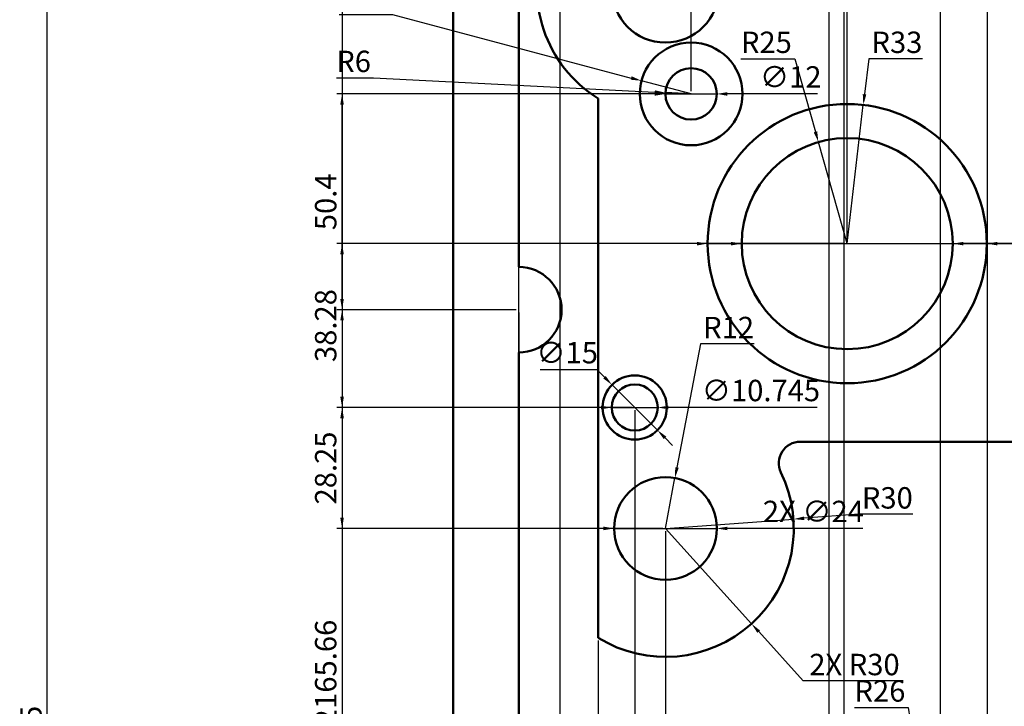
# Model space of a CAD drawing. Units: millimetres. Extents: x 1744 to 2162, y 1763 to 2334.
# Tile 3 of 5: x 1744 to 1975, y 2070 to 2230. Entities that reach past the tile are written whole.
import ezdxf

# ---------------------------------------------------------------- set-up
doc = ezdxf.new("R2010")
doc.units = ezdxf.units.MM
doc.layers.add('M-DIMS', color=2, linetype='Continuous', lineweight=25)
doc.layers.add('M-OUTL', color=7, linetype='Continuous', lineweight=50)
doc.styles.get("Standard").update_dxf_attribs({"font": 'arial.ttf'})
doc.dimstyles.new('ISO-25', dxfattribs={"dimtxt": 5, "dimasz": 2.5, "dimexe": 1.25, "dimexo": 0.625, "dimtad": 1, "dimtoh": 1, "dimdec": 0, "dimtxsty": 'Standard', "dimcen": 2.5, "dimadec": 0, "dimazin": 0, "dimtfac": 1, "dimtdec": 0, "dimtmove": 0, "dimatfit": 3, "dimfxl": 1, "dimarcsym": 0})

# ---------------------------------------------------------------- blocks, each defined once
blk = doc.blocks.new('*D1')
at = {"layer": 'Defpoints', "color": 0, "transparency": 16777216}
for p in [(1750.93, 2301.76), (1845.83, 2301.76), (1863.15, 1826.76)]:
    blk.add_point(p, dxfattribs=at)
at = {"layer": 'M-DIMS', "color": 0, "lineweight": -2, "transparency": 16777216}
for p, q in [((1845.2, 2301.76), (1749.68, 2301.76)), ((1750.93, 1829.26), (1750.93, 2299.26)), ((1862.52, 1826.76), (1749.68, 1826.76))]:
    blk.add_line(p, q, dxfattribs=at)
at = {"layer": 'M-DIMS', "color": 0, "transparency": 16777216}
for points in [[(1750.52, 2299.26), (1751.35, 2299.26), (1750.93, 2301.76)], [(1750.52, 1829.26), (1751.35, 1829.26), (1750.93, 1826.76)]]:
    blk.add_solid(points, dxfattribs=at)
at = {"layer": 'M-DIMS', "color": 0, "transparency": 16777216, "insert": (1747.76, 2064.26), "char_height": 5, "attachment_point": 5, "rotation": 90}
blk.add_mtext('475', dxfattribs=at)
blk = doc.blocks.new('*D8')
at = {"layer": 'Defpoints', "color": 0, "transparency": 16777216}
for p in [(1889.8, 2215.94), (1901.4, 2212.86)]:
    blk.add_point(p, dxfattribs=at)
at = {"layer": 'M-DIMS', "color": 0, "lineweight": -2, "transparency": 16777216}
for p, q in [((1819.12, 2231.4), (1831.64, 2231.4)), ((1831.64, 2231.4), (1887.38, 2216.58)), ((1901.4, 2212.86), (1889.8, 2215.94))]:
    blk.add_line(p, q, dxfattribs=at)
at = {"layer": 'M-DIMS', "color": 0, "transparency": 16777216}
blk.add_solid([(1887.49, 2216.99), (1887.28, 2216.18), (1889.8, 2215.94)], dxfattribs=at)
at = {"layer": 'M-DIMS', "color": 0, "transparency": 16777216, "insert": (1825.07, 2234.54), "char_height": 5, "attachment_point": 5}
blk.add_mtext('R12', dxfattribs=at)
blk = doc.blocks.new('*D9')
at = {"layer": 'Defpoints', "color": 0, "transparency": 16777216}
for p in [(1895.4, 2213.16), (1901.4, 2212.86)]:
    blk.add_point(p, dxfattribs=at)
at = {"layer": 'M-DIMS', "color": 0, "lineweight": -2, "transparency": 16777216}
for p, q in [((1818.49, 2216.64), (1827.18, 2216.64)), ((1827.18, 2216.64), (1892.91, 2213.29)), ((1901.4, 2212.86), (1895.4, 2213.16))]:
    blk.add_line(p, q, dxfattribs=at)
at = {"layer": 'M-DIMS', "color": 0, "transparency": 16777216}
blk.add_solid([(1892.93, 2213.71), (1892.89, 2212.87), (1895.4, 2213.16)], dxfattribs=at)
at = {"layer": 'M-DIMS', "color": 0, "transparency": 16777216, "insert": (1822.52, 2219.81), "char_height": 5, "attachment_point": 5}
blk.add_mtext('R6', dxfattribs=at)
blk = doc.blocks.new('*D10')
at = {"layer": 'Defpoints', "color": 0, "transparency": 16777216}
for p in [(1931.15, 2201.61), (1937.89, 2177.89)]:
    blk.add_point(p, dxfattribs=at)
at = {"layer": 'M-DIMS', "color": 0, "lineweight": -2, "transparency": 16777216}
for p, q in [((1913, 2221.09), (1925.61, 2221.09)), ((1925.61, 2221.09), (1930.47, 2204.01)), ((1937.89, 2177.89), (1931.15, 2201.61))]:
    blk.add_line(p, q, dxfattribs=at)
at = {"layer": 'M-DIMS', "color": 0, "transparency": 16777216}
blk.add_solid([(1930.87, 2204.12), (1930.06, 2203.9), (1931.15, 2201.61)], dxfattribs=at)
at = {"layer": 'M-DIMS', "color": 0, "transparency": 16777216, "insert": (1918.99, 2224.27), "char_height": 5, "attachment_point": 5}
blk.add_mtext('R25', dxfattribs=at)
blk = doc.blocks.new('*D11')
at = {"layer": 'Defpoints', "color": 0, "transparency": 16777216}
for p in [(1941.65, 2210.29), (1937.89, 2177.89)]:
    blk.add_point(p, dxfattribs=at)
at = {"layer": 'M-DIMS', "color": 0, "lineweight": -2, "transparency": 16777216}
for p, q in [((1942.9, 2221.09), (1941.93, 2212.77)), ((1955.47, 2221.09), (1942.9, 2221.09)), ((1937.89, 2177.89), (1941.65, 2210.29))]:
    blk.add_line(p, q, dxfattribs=at)
at = {"layer": 'M-DIMS', "color": 0, "transparency": 16777216}
blk.add_solid([(1941.52, 2212.82), (1942.35, 2212.72), (1941.65, 2210.29)], dxfattribs=at)
at = {"layer": 'M-DIMS', "color": 0, "transparency": 16777216, "insert": (1949.5, 2224.27), "char_height": 5, "attachment_point": 5}
blk.add_mtext('R33', dxfattribs=at)
blk = doc.blocks.new('*D12')
at = {"layer": 'Defpoints', "color": 0, "transparency": 16777216}
for p in [(1897.63, 2123.15), (1895.4, 2111.36)]:
    blk.add_point(p, dxfattribs=at)
at = {"layer": 'M-DIMS', "color": 0, "lineweight": -2, "transparency": 16777216}
for p, q in [((1903.58, 2154.51), (1898.1, 2125.6)), ((1916.1, 2154.51), (1903.58, 2154.51)), ((1895.4, 2111.36), (1897.63, 2123.15))]:
    blk.add_line(p, q, dxfattribs=at)
at = {"layer": 'M-DIMS', "color": 0, "transparency": 16777216}
blk.add_solid([(1897.69, 2125.68), (1898.51, 2125.53), (1897.63, 2123.15)], dxfattribs=at)
at = {"layer": 'M-DIMS', "color": 0, "transparency": 16777216, "insert": (1910.16, 2157.64), "char_height": 5, "attachment_point": 5}
blk.add_mtext('R12', dxfattribs=at)
blk = doc.blocks.new('*D13')
at = {"layer": 'Defpoints', "color": 0, "transparency": 16777216}
for p in [(1925.32, 2113.54), (1895.4, 2111.36)]:
    blk.add_point(p, dxfattribs=at)
at = {"layer": 'M-DIMS', "color": 0, "lineweight": -2, "transparency": 16777216}
for p, q in [((1895.4, 2111.36), (1925.32, 2113.54)), ((1940.67, 2114.67), (1927.81, 2113.73)), ((1953.23, 2114.67), (1940.67, 2114.67))]:
    blk.add_line(p, q, dxfattribs=at)
at = {"layer": 'M-DIMS', "color": 0, "transparency": 16777216}
blk.add_solid([(1927.78, 2114.14), (1927.84, 2113.31), (1925.32, 2113.54)], dxfattribs=at)
at = {"layer": 'M-DIMS', "color": 0, "transparency": 16777216, "insert": (1947.26, 2117.85), "char_height": 5, "attachment_point": 5}
blk.add_mtext('R30', dxfattribs=at)
blk = doc.blocks.new('*D15')
at = {"layer": 'Defpoints', "color": 0, "transparency": 16777216}
for p in [(1955.73, 2046.29), (1959.65, 2021.02)]:
    blk.add_point(p, dxfattribs=at)
at = {"layer": 'M-DIMS', "color": 0, "lineweight": -2, "transparency": 16777216}
for p, q in [((1939.55, 2069.57), (1952.12, 2069.57)), ((1952.12, 2069.57), (1955.35, 2048.77)), ((1959.65, 2021.02), (1955.73, 2046.29))]:
    blk.add_line(p, q, dxfattribs=at)
at = {"layer": 'M-DIMS', "color": 0, "transparency": 16777216}
blk.add_solid([(1955.76, 2048.83), (1954.94, 2048.7), (1955.73, 2046.29)], dxfattribs=at)
at = {"layer": 'M-DIMS', "color": 0, "transparency": 16777216, "insert": (1945.53, 2072.75), "char_height": 5, "attachment_point": 5}
blk.add_mtext('R26', dxfattribs=at)
blk = doc.blocks.new('*D29')
at = {"layer": 'Defpoints', "color": 0, "transparency": 16777216}
for p in [(2052.51, 2327.76), (2052.51, 1966.98), (1937.15, 1938.72)]:
    blk.add_point(p, dxfattribs=at)
at = {"layer": 'M-DIMS', "color": 0, "lineweight": -2, "transparency": 16777216}
for p, q in [((1937.15, 1939.34), (1937.15, 2329.01)), ((2052.51, 1967.6), (2052.51, 2329.01)), ((1939.65, 2327.76), (2050.01, 2327.76))]:
    blk.add_line(p, q, dxfattribs=at)
at = {"layer": 'M-DIMS', "color": 0, "transparency": 16777216}
for points in [[(1939.65, 2328.18), (1939.65, 2327.34), (1937.15, 2327.76)], [(2050.01, 2328.18), (2050.01, 2327.34), (2052.51, 2327.76)]]:
    blk.add_solid(points, dxfattribs=at)
at = {"layer": 'M-DIMS', "color": 0, "transparency": 16777216, "insert": (1994.83, 2330.94), "char_height": 5, "attachment_point": 5}
blk.add_mtext('115.35', dxfattribs=at)
blk = doc.blocks.new('*D30')
at = {"layer": 'Defpoints', "color": 0, "transparency": 16777216}
for p in [(1959.65, 2327.76), (1959.65, 2021.02), (1937.15, 1938.72)]:
    blk.add_point(p, dxfattribs=at)
at = {"layer": 'M-DIMS', "color": 0, "lineweight": -2, "transparency": 16777216}
for p, q in [((1937.15, 1939.34), (1937.15, 2329.01)), ((1959.65, 2021.64), (1959.65, 2329.01)), ((1939.65, 2327.76), (1957.15, 2327.76))]:
    blk.add_line(p, q, dxfattribs=at)
at = {"layer": 'M-DIMS', "color": 0, "transparency": 16777216}
for points in [[(1939.65, 2328.18), (1939.65, 2327.34), (1937.15, 2327.76)], [(1957.15, 2328.18), (1957.15, 2327.34), (1959.65, 2327.76)]]:
    blk.add_solid(points, dxfattribs=at)
at = {"layer": 'M-DIMS', "color": 0, "transparency": 16777216, "insert": (1948.4, 2330.94), "char_height": 5, "attachment_point": 5}
blk.add_mtext('22.5', dxfattribs=at)
blk = doc.blocks.new('*D34')
at = {"layer": 'Defpoints', "color": 0, "transparency": 16777216}
for p in [(2003.18, 2327.76), (2003.18, 2221.73), (1937.89, 2177.89)]:
    blk.add_point(p, dxfattribs=at)
at = {"layer": 'M-DIMS', "color": 0, "lineweight": -2, "transparency": 16777216}
for p, q in [((1937.89, 2178.51), (1937.89, 2329.01)), ((2003.18, 2222.36), (2003.18, 2329.01)), ((1940.39, 2327.76), (2000.68, 2327.76))]:
    blk.add_line(p, q, dxfattribs=at)
at = {"layer": 'M-DIMS', "color": 0, "transparency": 16777216}
for points in [[(1940.39, 2328.18), (1940.39, 2327.34), (1937.89, 2327.76)], [(2000.68, 2328.18), (2000.68, 2327.34), (2003.18, 2327.76)]]:
    blk.add_solid(points, dxfattribs=at)
at = {"layer": 'M-DIMS', "color": 0, "transparency": 16777216, "insert": (1970.53, 2330.94), "char_height": 5, "attachment_point": 5}
blk.add_mtext('65.29', dxfattribs=at)
blk = doc.blocks.new('*D36')
at = {"layer": 'Defpoints', "color": 0, "transparency": 16777216}
for p in [(1937.89, 2327.76), (1901.4, 2212.86), (1937.89, 2177.89)]:
    blk.add_point(p, dxfattribs=at)
at = {"layer": 'M-DIMS', "color": 0, "lineweight": -2, "transparency": 16777216}
for p, q in [((1901.4, 2213.48), (1901.4, 2329.01)), ((1937.89, 2178.51), (1937.89, 2329.01)), ((1903.9, 2327.76), (1935.39, 2327.76))]:
    blk.add_line(p, q, dxfattribs=at)
at = {"layer": 'M-DIMS', "color": 0, "transparency": 16777216}
for points in [[(1903.9, 2328.18), (1903.9, 2327.34), (1901.4, 2327.76)], [(1935.39, 2328.18), (1935.39, 2327.34), (1937.89, 2327.76)]]:
    blk.add_solid(points, dxfattribs=at)
at = {"layer": 'M-DIMS', "color": 0, "transparency": 16777216, "insert": (1919.64, 2330.94), "char_height": 5, "attachment_point": 5}
blk.add_mtext('36.49', dxfattribs=at)
blk = doc.blocks.new('*D37')
at = {"layer": 'Defpoints', "color": 0, "transparency": 16777216}
for p in [(1861.12, 2162.45), (1888.22, 2139.61), (1888.22, 1800.76)]:
    blk.add_point(p, dxfattribs=at)
at = {"layer": 'M-DIMS', "color": 0, "lineweight": -2, "transparency": 16777216}
for p, q in [((1861.12, 2161.83), (1861.12, 1799.51)), ((1888.22, 2138.98), (1888.22, 1799.51)), ((1863.62, 1800.76), (1885.72, 1800.76))]:
    blk.add_line(p, q, dxfattribs=at)
at = {"layer": 'M-DIMS', "color": 0, "transparency": 16777216}
for points in [[(1863.62, 1801.18), (1863.62, 1800.34), (1861.12, 1800.76)], [(1885.72, 1801.18), (1885.72, 1800.34), (1888.22, 1800.76)]]:
    blk.add_solid(points, dxfattribs=at)
at = {"layer": 'M-DIMS', "color": 0, "transparency": 16777216, "insert": (1874.67, 1803.9), "char_height": 5, "attachment_point": 5}
blk.add_mtext('27.1', dxfattribs=at)
blk = doc.blocks.new('*D39')
at = {"layer": 'Defpoints', "color": 0, "transparency": 16777216}
for p in [(1819.83, 2212.86), (1901.4, 2212.86), (1861.12, 2162.45)]:
    blk.add_point(p, dxfattribs=at)
at = {"layer": 'M-DIMS', "color": 0, "lineweight": -2, "transparency": 16777216}
for p, q in [((1900.77, 2212.86), (1818.58, 2212.86)), ((1819.83, 2164.95), (1819.83, 2210.36)), ((1860.5, 2162.45), (1818.58, 2162.45))]:
    blk.add_line(p, q, dxfattribs=at)
at = {"layer": 'M-DIMS', "color": 0, "transparency": 16777216}
for points in [[(1819.41, 2210.36), (1820.24, 2210.36), (1819.83, 2212.86)], [(1819.41, 2164.95), (1820.24, 2164.95), (1819.83, 2162.45)]]:
    blk.add_solid(points, dxfattribs=at)
at = {"layer": 'M-DIMS', "color": 0, "transparency": 16777216, "insert": (1816.65, 2187.66), "char_height": 5, "attachment_point": 5, "rotation": 90}
blk.add_mtext('50.4', dxfattribs=at)
blk = doc.blocks.new('*D40')
at = {"layer": 'Defpoints', "color": 0, "transparency": 16777216}
for p in [(1937.89, 2177.89), (2091.83, 2177.89), (2003.18, 2145.53)]:
    blk.add_point(p, dxfattribs=at)
at = {"layer": 'M-DIMS', "color": 0, "lineweight": -2, "transparency": 16777216}
for p, q in [((1938.51, 2177.89), (2093.08, 2177.89)), ((2091.83, 2148.03), (2091.83, 2175.39)), ((2003.8, 2145.53), (2093.08, 2145.53))]:
    blk.add_line(p, q, dxfattribs=at)
at = {"layer": 'M-DIMS', "color": 0, "transparency": 16777216}
for points in [[(2091.41, 2175.39), (2092.24, 2175.39), (2091.83, 2177.89)], [(2091.41, 2148.03), (2092.24, 2148.03), (2091.83, 2145.53)]]:
    blk.add_solid(points, dxfattribs=at)
at = {"layer": 'M-DIMS', "color": 0, "transparency": 16777216, "insert": (2088.65, 2161.71), "char_height": 5, "attachment_point": 5, "rotation": 90}
blk.add_mtext('32.36', dxfattribs=at)
blk = doc.blocks.new('*D41')
at = {"layer": 'Defpoints', "color": 0, "transparency": 16777216}
for p in [(1937.89, 2177.89), (1819.83, 2139.61), (1888.22, 2139.61)]:
    blk.add_point(p, dxfattribs=at)
at = {"layer": 'M-DIMS', "color": 0, "lineweight": -2, "transparency": 16777216}
for p, q in [((1937.26, 2177.89), (1818.58, 2177.89)), ((1819.83, 2175.39), (1819.83, 2142.11)), ((1887.6, 2139.61), (1818.58, 2139.61))]:
    blk.add_line(p, q, dxfattribs=at)
at = {"layer": 'M-DIMS', "color": 0, "transparency": 16777216}
for points in [[(1819.41, 2175.39), (1820.24, 2175.39), (1819.83, 2177.89)], [(1819.41, 2142.11), (1820.24, 2142.11), (1819.83, 2139.61)]]:
    blk.add_solid(points, dxfattribs=at)
at = {"layer": 'M-DIMS', "color": 0, "transparency": 16777216, "insert": (1816.65, 2158.75), "char_height": 5, "attachment_point": 5, "rotation": 90}
blk.add_mtext('38.28', dxfattribs=at)
blk = doc.blocks.new('*D42')
at = {"layer": 'Defpoints', "color": 0, "transparency": 16777216}
for p in [(1888.22, 2139.61), (1819.83, 2111.36), (1895.4, 2111.36)]:
    blk.add_point(p, dxfattribs=at)
at = {"layer": 'M-DIMS', "color": 0, "lineweight": -2, "transparency": 16777216}
for p, q in [((1887.6, 2139.61), (1818.58, 2139.61)), ((1819.83, 2137.11), (1819.83, 2113.86)), ((1894.77, 2111.36), (1818.58, 2111.36))]:
    blk.add_line(p, q, dxfattribs=at)
at = {"layer": 'M-DIMS', "color": 0, "transparency": 16777216}
for points in [[(1819.41, 2137.11), (1820.24, 2137.11), (1819.83, 2139.61)], [(1819.41, 2113.86), (1820.24, 2113.86), (1819.83, 2111.36)]]:
    blk.add_solid(points, dxfattribs=at)
at = {"layer": 'M-DIMS', "color": 0, "transparency": 16777216, "insert": (1816.65, 2125.48), "char_height": 5, "attachment_point": 5, "rotation": 90}
blk.add_mtext('28.25', dxfattribs=at)
blk = doc.blocks.new('*D46')
at = {"layer": 'Defpoints', "color": 0, "transparency": 16777216}
for p in [(2052.51, 2327.76), (1861.12, 1859.18), (2052.51, 1857.29)]:
    blk.add_point(p, dxfattribs=at)
at = {"layer": 'M-DIMS', "color": 0, "lineweight": -2, "transparency": 16777216}
for p, q in [((1861.12, 1859.81), (1861.12, 2329.01)), ((2052.51, 1857.91), (2052.51, 2329.01)), ((1863.62, 2327.76), (2050.01, 2327.76))]:
    blk.add_line(p, q, dxfattribs=at)
at = {"layer": 'M-DIMS', "color": 0, "transparency": 16777216}
for points in [[(1863.62, 2328.18), (1863.62, 2327.34), (1861.12, 2327.76)], [(2050.01, 2328.18), (2050.01, 2327.34), (2052.51, 2327.76)]]:
    blk.add_solid(points, dxfattribs=at)
at = {"layer": 'M-DIMS', "color": 0, "transparency": 16777216, "insert": (1956.82, 2330.94), "char_height": 5, "attachment_point": 5}
blk.add_mtext('191.4', dxfattribs=at)
blk = doc.blocks.new('*D47')
at = {"layer": 'Defpoints', "color": 0, "transparency": 16777216}
for p in [(1871.12, 2284.44), (1819.83, 1842.43), (1870.79, 1842.43)]:
    blk.add_point(p, dxfattribs=at)
at = {"layer": 'M-DIMS', "color": 0, "lineweight": -2, "transparency": 16777216}
for p, q in [((1870.5, 2284.44), (1818.58, 2284.44)), ((1819.83, 2281.94), (1819.83, 1844.93)), ((1870.17, 1842.43), (1818.58, 1842.43))]:
    blk.add_line(p, q, dxfattribs=at)
at = {"layer": 'M-DIMS', "color": 0, "transparency": 16777216}
for points in [[(1819.41, 2281.94), (1820.24, 2281.94), (1819.83, 2284.44)], [(1819.41, 1844.93), (1820.24, 1844.93), (1819.83, 1842.43)]]:
    blk.add_solid(points, dxfattribs=at)
at = {"layer": 'M-DIMS', "color": 0, "transparency": 16777216, "insert": (1816.69, 2063.44), "char_height": 5, "attachment_point": 5, "rotation": 90}
blk.add_mtext('442', dxfattribs=at)
blk = doc.blocks.new('*D48')
at = {"layer": 'Defpoints', "color": 0, "transparency": 16777216}
for p in [(1861.12, 2327.76), (1861.12, 1859.18), (1845.83, 1856.76)]:
    blk.add_point(p, dxfattribs=at)
at = {"layer": 'M-DIMS', "color": 0, "lineweight": -2, "transparency": 16777216}
for p, q in [((1845.83, 1857.39), (1845.83, 2329.01)), ((1861.12, 1859.81), (1861.12, 2329.01)), ((1848.33, 2327.76), (1858.62, 2327.76)), ((1861.12, 2327.76), (1885.17, 2327.76))]:
    blk.add_line(p, q, dxfattribs=at)
at = {"layer": 'M-DIMS', "color": 0, "transparency": 16777216}
for points in [[(1848.33, 2328.18), (1848.33, 2327.34), (1845.83, 2327.76)], [(1858.62, 2328.18), (1858.62, 2327.34), (1861.12, 2327.76)]]:
    blk.add_solid(points, dxfattribs=at)
at = {"layer": 'M-DIMS', "color": 0, "transparency": 16777216, "insert": (1874.4, 2330.94), "char_height": 5, "attachment_point": 5}
blk.add_mtext('15.298', dxfattribs=at)
blk = doc.blocks.new('*D53')
at = {"layer": 'Defpoints', "color": 0, "transparency": 16777216}
for p in [(1861.12, 2162.45), (1819.83, 1996.79), (1861.12, 1996.79)]:
    blk.add_point(p, dxfattribs=at)
at = {"layer": 'M-DIMS', "color": 0, "lineweight": -2, "transparency": 16777216}
for p, q in [((1860.5, 2162.45), (1818.58, 2162.45)), ((1819.83, 2159.95), (1819.83, 1999.29)), ((1860.5, 1996.79), (1818.58, 1996.79))]:
    blk.add_line(p, q, dxfattribs=at)
at = {"layer": 'M-DIMS', "color": 0, "transparency": 16777216}
for points in [[(1819.41, 2159.95), (1820.24, 2159.95), (1819.83, 2162.45)], [(1819.41, 1999.29), (1820.24, 1999.29), (1819.83, 1996.79)]]:
    blk.add_solid(points, dxfattribs=at)
at = {"layer": 'M-DIMS', "color": 0, "transparency": 16777216, "insert": (1816.65, 2079.62), "char_height": 5, "attachment_point": 5, "rotation": 90}
blk.add_mtext('165.66', dxfattribs=at)
blk = doc.blocks.new('*D60')
at = {"layer": 'Defpoints', "color": 0, "transparency": 16777216}
for p in [(1933.69, 2327.76), (1870.79, 1842.43), (1933.69, 1842.43)]:
    blk.add_point(p, dxfattribs=at)
at = {"layer": 'M-DIMS', "color": 0, "lineweight": -2, "transparency": 16777216}
for p, q in [((1870.79, 1843.06), (1870.79, 2329.01)), ((1933.69, 1843.06), (1933.69, 2329.01)), ((1873.29, 2327.76), (1931.19, 2327.76))]:
    blk.add_line(p, q, dxfattribs=at)
at = {"layer": 'M-DIMS', "color": 0, "transparency": 16777216}
for points in [[(1873.29, 2328.18), (1873.29, 2327.34), (1870.79, 2327.76)], [(1931.19, 2328.18), (1931.19, 2327.34), (1933.69, 2327.76)]]:
    blk.add_solid(points, dxfattribs=at)
at = {"layer": 'M-DIMS', "color": 0, "transparency": 16777216, "insert": (1902.24, 2330.94), "char_height": 5, "attachment_point": 5}
blk.add_mtext('62.9', dxfattribs=at)
blk = doc.blocks.new('*D61')
at = {"layer": 'Defpoints', "color": 0, "transparency": 16777216}
for p in [(1970.69, 2327.76), (1933.69, 1842.43), (1970.69, 1842.43)]:
    blk.add_point(p, dxfattribs=at)
at = {"layer": 'M-DIMS', "color": 0, "lineweight": -2, "transparency": 16777216}
for p, q in [((1933.69, 1843.06), (1933.69, 2329.01)), ((1970.69, 1843.06), (1970.69, 2329.01)), ((1936.19, 2327.76), (1968.19, 2327.76))]:
    blk.add_line(p, q, dxfattribs=at)
at = {"layer": 'M-DIMS', "color": 0, "transparency": 16777216}
for points in [[(1936.19, 2328.18), (1936.19, 2327.34), (1933.69, 2327.76)], [(1968.19, 2328.18), (1968.19, 2327.34), (1970.69, 2327.76)]]:
    blk.add_solid(points, dxfattribs=at)
at = {"layer": 'M-DIMS', "color": 0, "transparency": 16777216, "insert": (1952.19, 2330.94), "char_height": 5, "attachment_point": 5}
blk.add_mtext('37', dxfattribs=at)
blk = doc.blocks.new('*D67')
at = {"layer": 'Defpoints', "color": 0, "transparency": 16777216}
for p in [(1861.12, 2162.45), (1895.4, 2111.36), (1895.4, 1800.76)]:
    blk.add_point(p, dxfattribs=at)
at = {"layer": 'M-DIMS', "color": 0, "lineweight": -2, "transparency": 16777216}
for p, q in [((1861.12, 2161.83), (1861.12, 1799.51)), ((1895.4, 2110.73), (1895.4, 1799.51)), ((1863.62, 1800.76), (1892.9, 1800.76))]:
    blk.add_line(p, q, dxfattribs=at)
at = {"layer": 'M-DIMS', "color": 0, "transparency": 16777216}
for points in [[(1863.62, 1801.18), (1863.62, 1800.34), (1861.12, 1800.76)], [(1892.9, 1801.18), (1892.9, 1800.34), (1895.4, 1800.76)]]:
    blk.add_solid(points, dxfattribs=at)
at = {"layer": 'M-DIMS', "color": 0, "transparency": 16777216, "insert": (1878.26, 1803.94), "char_height": 5, "attachment_point": 5}
blk.add_mtext('34.273', dxfattribs=at)
blk = doc.blocks.new('*D69')
at = {"layer": 'Defpoints', "color": 0, "transparency": 16777216}
for p in [(1861.12, 2162.45), (1879.67, 2085.81), (1861.12, 1800.76)]:
    blk.add_point(p, dxfattribs=at)
at = {"layer": 'M-DIMS', "color": 0, "lineweight": -2, "transparency": 16777216}
for p, q in [((1861.12, 2161.83), (1861.12, 1799.51)), ((1879.67, 2085.19), (1879.67, 1799.51)), ((1877.17, 1800.76), (1863.62, 1800.76))]:
    blk.add_line(p, q, dxfattribs=at)
at = {"layer": 'M-DIMS', "color": 0, "transparency": 16777216}
for points in [[(1863.62, 1801.18), (1863.62, 1800.34), (1861.12, 1800.76)], [(1877.17, 1801.18), (1877.17, 1800.34), (1879.67, 1800.76)]]:
    blk.add_solid(points, dxfattribs=at)
at = {"layer": 'M-DIMS', "color": 0, "transparency": 16777216, "insert": (1870.39, 1803.94), "char_height": 5, "attachment_point": 5}
blk.add_mtext('18.54', dxfattribs=at)
blk = doc.blocks.new('*D74')
at = {"layer": 'Defpoints', "color": 0, "transparency": 16777216}
for p in [(1882.92, 2144.91), (1893.53, 2134.31)]:
    blk.add_point(p, dxfattribs=at)
at = {"layer": 'M-DIMS', "color": 0, "lineweight": -2, "transparency": 16777216}
for p, q in [((1866.12, 2148.45), (1879.38, 2148.45)), ((1879.38, 2148.45), (1881.15, 2146.68)), ((1893.53, 2134.31), (1882.92, 2144.91)), ((1895.3, 2132.54), (1897.06, 2130.77))]:
    blk.add_line(p, q, dxfattribs=at)
at = {"layer": 'M-DIMS', "color": 0, "transparency": 16777216}
for points in [[(1881.45, 2146.97), (1880.86, 2146.39), (1882.92, 2144.91)], [(1895.59, 2132.83), (1895, 2132.24), (1893.53, 2134.31)]]:
    blk.add_solid(points, dxfattribs=at)
at = {"layer": 'M-DIMS', "color": 0, "transparency": 16777216, "insert": (1872.44, 2151.77), "char_height": 5, "attachment_point": 5}
blk.add_mtext('∅15', dxfattribs=at)
blk = doc.blocks.new('*D75')
at = {"layer": 'Defpoints', "color": 0, "transparency": 16777216}
for p in [(1882.85, 2139.61), (1893.6, 2139.61)]:
    blk.add_point(p, dxfattribs=at)
at = {"layer": 'M-DIMS', "color": 0, "lineweight": -2, "transparency": 16777216}
for p, q in [((1880.35, 2139.61), (1877.85, 2139.61)), ((1882.85, 2139.61), (1893.6, 2139.61)), ((1903.98, 2139.61), (1896.1, 2139.61)), ((1930.84, 2139.61), (1903.98, 2139.61))]:
    blk.add_line(p, q, dxfattribs=at)
at = {"layer": 'M-DIMS', "color": 0, "transparency": 16777216}
for points in [[(1880.35, 2140.03), (1880.35, 2139.19), (1882.85, 2139.61)], [(1896.1, 2140.03), (1896.1, 2139.19), (1893.6, 2139.61)]]:
    blk.add_solid(points, dxfattribs=at)
at = {"layer": 'M-DIMS', "color": 0, "transparency": 16777216, "insert": (1917.72, 2142.93), "char_height": 5, "attachment_point": 5}
blk.add_mtext('∅10.745', dxfattribs=at)
blk = doc.blocks.new('*D79')
at = {"layer": 'Defpoints', "color": 0, "transparency": 16777216}
for p in [(1905.27, 2177.89), (1970.5, 2177.89)]:
    blk.add_point(p, dxfattribs=at)
at = {"layer": 'M-DIMS', "color": 0, "lineweight": -2, "transparency": 16777216}
for p, q in [((1902.77, 2177.89), (1900.27, 2177.89)), ((1905.27, 2177.89), (1970.5, 2177.89)), ((1990.07, 2177.89), (1973, 2177.89)), ((2012.99, 2177.89), (1990.07, 2177.89))]:
    blk.add_line(p, q, dxfattribs=at)
at = {"layer": 'M-DIMS', "color": 0, "transparency": 16777216}
for points in [[(1902.77, 2178.3), (1902.77, 2177.47), (1905.27, 2177.89)], [(1973, 2178.3), (1973, 2177.47), (1970.5, 2177.89)]]:
    blk.add_solid(points, dxfattribs=at)
at = {"layer": 'M-DIMS', "color": 0, "transparency": 16777216, "insert": (2001.84, 2181.21), "char_height": 5, "attachment_point": 5}
blk.add_mtext('∅65.24', dxfattribs=at)
blk = doc.blocks.new('*D80')
at = {"layer": 'Defpoints', "color": 0, "transparency": 16777216}
for p in [(1895.4, 2111.36), (1915.51, 2089.1)]:
    blk.add_point(p, dxfattribs=at)
at = {"layer": 'M-DIMS', "color": 0, "lineweight": -2, "transparency": 16777216}
for p, q in [((1895.4, 2111.36), (1915.51, 2089.1)), ((1927.58, 2075.74), (1917.19, 2087.25)), ((1950.96, 2075.74), (1927.58, 2075.74))]:
    blk.add_line(p, q, dxfattribs=at)
at = {"layer": 'M-DIMS', "color": 0, "transparency": 16777216}
blk.add_solid([(1917.5, 2087.52), (1916.88, 2086.97), (1915.51, 2089.1)], dxfattribs=at)
at = {"layer": 'M-DIMS', "color": 0, "transparency": 16777216, "insert": (1939.58, 2078.92), "char_height": 5, "attachment_point": 5}
blk.add_mtext('2X R30', dxfattribs=at)
blk = doc.blocks.new('*D82')
at = {"layer": 'Defpoints', "color": 0, "transparency": 16777216}
for p in [(1913.23, 2177.89), (1962.54, 2177.89)]:
    blk.add_point(p, dxfattribs=at)
at = {"layer": 'M-DIMS', "color": 0, "lineweight": -2, "transparency": 16777216}
for p, q in [((1910.73, 2177.89), (1908.23, 2177.89)), ((1913.23, 2177.89), (1962.54, 2177.89)), ((1977.34, 2177.89), (1965.04, 2177.89)), ((1999.31, 2177.89), (1977.34, 2177.89))]:
    blk.add_line(p, q, dxfattribs=at)
at = {"layer": 'M-DIMS', "color": 0, "transparency": 16777216}
for points in [[(1910.73, 2178.3), (1910.73, 2177.47), (1913.23, 2177.89)], [(1965.04, 2178.3), (1965.04, 2177.47), (1962.54, 2177.89)]]:
    blk.add_solid(points, dxfattribs=at)
at = {"layer": 'M-DIMS', "color": 0, "transparency": 16777216, "insert": (1988.63, 2181.21), "char_height": 5, "attachment_point": 5}
blk.add_mtext('∅49.31', dxfattribs=at)
blk = doc.blocks.new('*D86')
at = {"layer": 'Defpoints', "color": 0, "transparency": 16777216}
for p in [(1883.4, 2111.36), (1907.4, 2111.36)]:
    blk.add_point(p, dxfattribs=at)
at = {"layer": 'M-DIMS', "color": 0, "lineweight": -2, "transparency": 16777216}
for p, q in [((1880.9, 2111.36), (1878.4, 2111.36)), ((1883.4, 2111.36), (1907.4, 2111.36)), ((1917.78, 2111.36), (1909.9, 2111.36)), ((1941.55, 2111.36), (1917.78, 2111.36))]:
    blk.add_line(p, q, dxfattribs=at)
at = {"layer": 'M-DIMS', "color": 0, "transparency": 16777216}
for points in [[(1880.9, 2111.78), (1880.9, 2110.94), (1883.4, 2111.36)], [(1909.9, 2111.77), (1909.9, 2110.94), (1907.4, 2111.36)]]:
    blk.add_solid(points, dxfattribs=at)
at = {"layer": 'M-DIMS', "color": 0, "transparency": 16777216, "insert": (1929.98, 2114.68), "char_height": 5, "attachment_point": 5}
blk.add_mtext('2X ∅24', dxfattribs=at)
blk = doc.blocks.new('*D89')
at = {"layer": 'Defpoints', "color": 0, "transparency": 16777216}
for p in [(1895.4, 2212.86), (1907.4, 2212.86)]:
    blk.add_point(p, dxfattribs=at)
at = {"layer": 'M-DIMS', "color": 0, "lineweight": -2, "transparency": 16777216}
for p, q in [((1892.9, 2212.86), (1890.4, 2212.86)), ((1895.4, 2212.86), (1907.4, 2212.86)), ((1917.78, 2212.86), (1909.9, 2212.86)), ((1930.96, 2212.86), (1917.78, 2212.86))]:
    blk.add_line(p, q, dxfattribs=at)
at = {"layer": 'M-DIMS', "color": 0, "transparency": 16777216}
for points in [[(1892.9, 2213.28), (1892.9, 2212.44), (1895.4, 2212.86)], [(1909.9, 2213.27), (1909.9, 2212.44), (1907.4, 2212.86)]]:
    blk.add_solid(points, dxfattribs=at)
at = {"layer": 'M-DIMS', "color": 0, "transparency": 16777216, "insert": (1924.68, 2216.18), "char_height": 5, "attachment_point": 5}
blk.add_mtext('∅12', dxfattribs=at)

msp = doc.modelspace()

# ---------------------------------------------------------------- linework, layer by layer
at = {"layer": 'M-OUTL'}
for p, q in [((1845.8255, 2301.7604), (1845.8255, 1856.7604)), ((1861.1237, 2274.4372), (1861.1237, 2172.4535)), ((1879.6653, 2176.284), (1879.6653, 2211.814)), ((1879.6653, 2176.284), (1879.6653, 2085.814)), ((1861.1237, 2152.4535), (1861.1237, 2006.7886)), ((1926.8997, 2131.6094), (1930.1843, 2131.6094)), ((1930.1843, 2131.6094), (2015.2647, 2131.6094))]:
    msp.add_line(p, q, dxfattribs=at)
for centre, radius in [((1895.3972, 2237.3582), 12.5), ((1901.3972, 2212.8582), 12), ((1901.3972, 2212.8582), 6), ((1937.8856, 2177.888), 32.6177), ((1937.8856, 2177.888), 24.6559), ((1888.2243, 2139.6094), 7.5002), ((1888.2243, 2139.6094), 5.3724), ((1895.3972, 2111.3582), 12)]:
    msp.add_circle(centre, radius, dxfattribs=at)
for centre, radius, start, end in [((1895.3972, 2237.3582), 30, 0, 238.372386), ((1861.1237, 2162.4535), 10, 270, 90), ((1926.8997, 2126.6094), 5, 90, 205.832786), ((1895.3972, 2111.3582), 30, 238.372386, 25.832786)]:
    msp.add_arc(centre, radius, start, end, dxfattribs=at)

# ---------------------------------------------------------------- dimensions: what is measured, and where the dimension line sits
at = {"layer": 'M-DIMS'}
for base, p1, p2, override, picture, middle in [((1861.1237, 2327.7604), (1845.8255, 1856.7604), (1861.1237, 1859.184), {"dimdec": 3, "dimlfac": 1, "dimrnd": 0, "dimzin": 0, "dimdsep": 46, "dimlunit": 2}, '*D48', (1874.3971, 2330.9382)), ((2052.5068, 2327.7604), (1861.1237, 1859.184), (2052.5068, 1857.2889), {"dimdec": 1, "dimlfac": 1, "dimrnd": 0, "dimzin": 0, "dimdsep": 46, "dimlunit": 2}, '*D46', (1956.8153, 2330.9382)), ((1933.6942, 2327.7604), (1870.7949, 1842.4331), (1933.6942, 1842.4331), {"dimdec": 1, "dimlfac": 1, "dimrnd": 0, "dimzin": 0, "dimdsep": 46, "dimlunit": 2}, '*D60', (1902.2445, 2330.9382)), ((1937.8856, 2327.7604), (1901.3972, 2212.8582), (1937.8856, 2177.888), {"dimdec": 2, "dimlfac": 1, "dimrnd": 0, "dimzin": 0, "dimdsep": 46, "dimlunit": 2}, '*D36', (1919.6414, 2330.9399)), ((1970.6942, 2327.7604), (1933.6942, 1842.4331), (1970.6942, 1842.4331), {"dimdec": 0, "dimlfac": 1, "dimrnd": 0, "dimzin": 0, "dimdsep": 46, "dimlunit": 2}, '*D61', (1952.1942, 2330.9399)), ((2052.5068, 2327.7604), (1937.1543, 1938.7171), (2052.5068, 1966.9753), {"dimdec": 2, "dimlfac": 1, "dimrnd": 0, "dimzin": 0, "dimdsep": 46, "dimlunit": 2}, '*D29', (1994.8306, 2330.9399)), ((1959.6543, 2327.7604), (1937.1543, 1938.7171), (1959.6543, 2021.0157), {"dimdec": 1, "dimlfac": 1, "dimrnd": 0, "dimzin": 0, "dimdsep": 46, "dimlunit": 2}, '*D30', (1948.4043, 2330.9382)), ((2003.178, 2327.7604), (1937.8856, 2177.888), (2003.178, 2221.7343), {"dimdec": 2, "dimlfac": 1, "dimrnd": 0, "dimzin": 0, "dimdsep": 46, "dimlunit": 2}, '*D34', (1970.5318, 2330.9382)), ((1888.2243, 1800.7604), (1861.1237, 2162.4535), (1888.2243, 2139.6094), {"dimdec": 1, "dimlfac": 1, "dimrnd": 0, "dimzin": 0, "dimdsep": 46, "dimlunit": 2}, '*D37', (1874.674, 1803.8956)), ((1895.39722, 1800.76037), (1861.12374, 2162.45354), (1895.39722, 2111.35824), {"dimdec": 3, "dimlfac": 1, "dimrnd": 0, "dimzin": 0, "dimdsep": 46, "dimlunit": 2}, '*D67', (1878.26048, 1803.93994)), ((1861.1237, 1800.7604), (1879.6653, 2085.814), (1861.1237, 2162.4535), {"dimdec": 2, "dimlfac": 1, "dimrnd": 0, "dimzin": 0, "dimdsep": 46, "dimlunit": 2}, '*D69', (1870.3945, 1803.9382))]:
    dim = msp.add_linear_dim(base=base, p1=p1, p2=p2, dimstyle='ISO-25', override=override, dxfattribs=at)
    dim.commit()
    dim.dimension.update_dxf_attribs({"geometry": picture, "text_midpoint": middle})
for base, p1, p2, override, picture, middle in [((1750.9321, 2301.7604), (1863.146, 1826.7604), (1845.8255, 2301.7604), {"dimclrd": 0, "dimclre": 0, "dimclrt": 0}, '*D1', (1747.7645, 2064.2604)), ((1819.8255, 1842.4331), (1871.1237, 2284.4372), (1870.7949, 1842.4331), {"dimdec": 0, "dimlfac": 1, "dimrnd": 0, "dimzin": 0, "dimdsep": 46, "dimlunit": 2}, '*D47', (1816.6902, 2063.4352)), ((1819.8255, 2212.8582), (1861.1237, 2162.4535), (1901.3972, 2212.8582), {"dimdec": 1, "dimlfac": 1, "dimrnd": 0, "dimzin": 0, "dimdsep": 46, "dimlunit": 2}, '*D39', (1816.6476, 2187.6559)), ((1819.8255, 2139.6094), (1937.8856, 2177.888), (1888.2243, 2139.6094), {"dimdec": 2, "dimlfac": 1, "dimrnd": 0, "dimzin": 0, "dimdsep": 46, "dimlunit": 2}, '*D41', (1816.6459, 2158.7487)), ((2091.8255, 2177.888), (2003.178, 2145.5271), (1937.8856, 2177.888), {"dimdec": 2, "dimlfac": 1, "dimrnd": 0, "dimzin": 0, "dimdsep": 46, "dimlunit": 2}, '*D40', (2088.6459, 2161.7076)), ((1819.8255, 1996.7886), (1861.1237, 2162.4535), (1861.1237, 1996.7886), {"dimdec": 2, "dimlfac": 1, "dimrnd": 0, "dimzin": 0, "dimdsep": 46, "dimlunit": 2}, '*D53', (1816.6476, 2079.621)), ((1819.8255, 2111.3582), (1888.2243, 2139.6094), (1895.3972, 2111.3582), {"dimdec": 2, "dimlfac": 1, "dimrnd": 0, "dimzin": 0, "dimdsep": 46, "dimlunit": 2}, '*D42', (1816.6476, 2125.4838))]:
    dim = msp.add_linear_dim(base=base, p1=p1, p2=p2, angle=90, dimstyle='ISO-25', override=override, dxfattribs=at)
    dim.commit()
    dim.dimension.update_dxf_attribs({"geometry": picture, "text_midpoint": middle})
for center, mpoint, picture, middle in [((1901.3972, 2212.8582), (1889.8, 2215.9412), '*D8', (1831.6392, 2231.4026)), ((1937.8856, 2177.888), (1931.1483, 2201.6055), '*D10', (1918.9948, 2221.0941)), ((1937.8856, 2177.888), (1941.6467, 2210.2881), '*D11', (1949.4998, 2221.0941)), ((1901.3972, 2212.8582), (1895.405, 2213.1633), '*D9', (1827.1776, 2216.6364)), ((1895.3972, 2111.3582), (1897.6339, 2123.148), '*D12', (1910.1561, 2154.5068)), ((1895.3972, 2111.3582), (1925.3175, 2113.5442), '*D13', (1940.6703, 2114.6659)), ((1959.6543, 2021.0157), (1955.7334, 2046.2948), '*D15', (1945.5266, 2069.568))]:
    dim = msp.add_radius_dim(center=center, mpoint=mpoint, dimstyle='ISO-25', override={"dimclrd": 0, "dimclre": 0, "dimclrt": 0}, dxfattribs=at)
    dim.commit()
    dim.dimension.update_dxf_attribs({"geometry": picture, "text_midpoint": middle, "dimtype": 164})
for p1, p2, override, picture, middle in [((1895.3972, 2212.8585), (1907.3972, 2212.858), {"dimdec": 0, "dimlfac": 1, "dimrnd": 0, "dimzin": 0, "dimdsep": 46, "dimlunit": 2}, '*D89', (1917.7826, 2212.8576)), ((1905.268, 2177.8879), (1970.5033, 2177.888), {"dimdec": 2, "dimlfac": 1, "dimrnd": 0, "dimzin": 0, "dimdsep": 46, "dimlunit": 2}, '*D79', (1990.0739, 2177.888)), ((1913.2298, 2177.8879), (1962.5415, 2177.888), {"dimdec": 2, "dimlfac": 1, "dimrnd": 0, "dimzin": 0, "dimdsep": 46, "dimlunit": 2}, '*D82', (1977.335, 2177.888)), ((1893.5281, 2134.3064), (1882.9205, 2144.9125), {"dimdec": 0, "dimlfac": 1, "dimrnd": 0, "dimzin": 0, "dimdsep": 46, "dimlunit": 2}, '*D74', (1872.4398, 2148.4477)), ((1882.8519, 2139.6099), (1893.5968, 2139.609), {"dimdec": 3, "dimlfac": 1, "dimrnd": 0, "dimzin": 0, "dimdsep": 46, "dimlunit": 2}, '*D75', (1903.9822, 2139.6081))]:
    dim = msp.add_diameter_dim_2p(p1=p1, p2=p2, dimstyle='ISO-25', override=override, dxfattribs=at)
    dim.commit()
    dim.dimension.update_dxf_attribs({"geometry": picture, "text_midpoint": middle, "dimtype": 163})
dim = msp.add_diameter_dim_2p(p1=(1883.3972, 2111.3585), p2=(1907.3972, 2111.358), text='2X <>', dimstyle='ISO-25', override={"dimdec": 0, "dimlfac": 1, "dimrnd": 0, "dimzin": 0, "dimdsep": 46, "dimlunit": 2}, dxfattribs=at)
dim.commit()
dim.dimension.update_dxf_attribs({"geometry": '*D86', "text_midpoint": (1917.7826, 2111.3578), "dimtype": 163})
dim = msp.add_radius_dim(center=(1895.3972, 2111.3582), mpoint=(1915.5111, 2089.0999), text='2X <>', dimstyle='ISO-25', override={"dimdec": 0, "dimlfac": 1, "dimrnd": 0, "dimzin": 0, "dimdsep": 46, "dimlunit": 2}, dxfattribs=at)
dim.commit()
dim.dimension.update_dxf_attribs({"geometry": '*D80', "text_midpoint": (1939.584, 2075.7449), "dimtype": 164})

doc.saveas('drawing.dxf')
